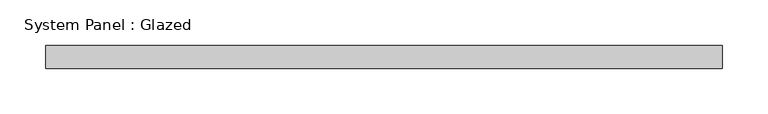
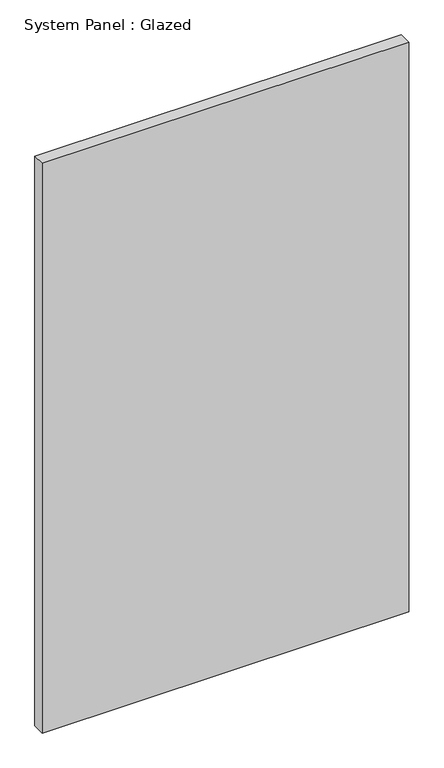
"""IFC4 building model written with IfcOpenShell, lengths in millimetres: plate geometry, System Panel : Glazed."""

from ifc_helpers import new_model, si_unit, origin, origin_with_axes, place, context, project, spatial, polyline, outline, extrude, source, transform, mapped, element, save


def system_panel_glazed_204414d1(model_context):
    return source(origin(), model_context, "Body", "SweptSolid", [
        extrude(outline(polyline([(371.475, 19.05), (-371.475, 19.05), (-371.475, 44.45), (371.475, 44.45), (371.475, 19.05)])), origin_with_axes(), (0.0, 0.0, 1.0), 1220.9161516),
    ])


if __name__ == "__main__":
    model = new_model("IFC4")
    model_context = context("Model", 3, world=origin())
    ifc_project = project(units=[si_unit("LENGTHUNIT", "METRE", prefix="MILLI")], contexts=[model_context])
    site = spatial("IfcSite", under=ifc_project)
    building = spatial("IfcBuilding", under=site)
    placement = place(None, origin())
    system_panel_glazed_shape = system_panel_glazed_204414d1(model_context)
    element("IfcPlate", 1, ObjectType="System Panel : Glazed", at=placement, inside=building, context=model_context, shape_type="MappedRepresentation", body=[
        mapped(system_panel_glazed_shape, transform((0.0, 0.0, 0.0), x_axis=(1.0, 0.0, 0.0), y_axis=(0.0, 1.0, 0.0), z_axis=(0.0, 0.0, 1.0))),
    ])
    save(model, "model.ifc")

# Revit data of these elements
# Type "System Panel : Glazed"
#   Construction Type Id = "GSP4R"
#   Analytic Construction = "1/8 in Pilkington single glazing"
#   Visual Light Transmittance = 0.9
#   Solar Heat Gain Coefficient = 0.86
#   Heat Transfer Coefficient (U) = 1.18115 BTU/(h·ft²·°F)
#   Define Thermal Properties by = 1
# Element 1 (IfcPlate, "System Panel : Glazed")
#   Materials on its faces: "Glass"
# Materials
#   "Glass": class "Glass", colour RGB 0 128 192, transparency 0.75, Description = "Soda Lime Glass", Cost = 0
